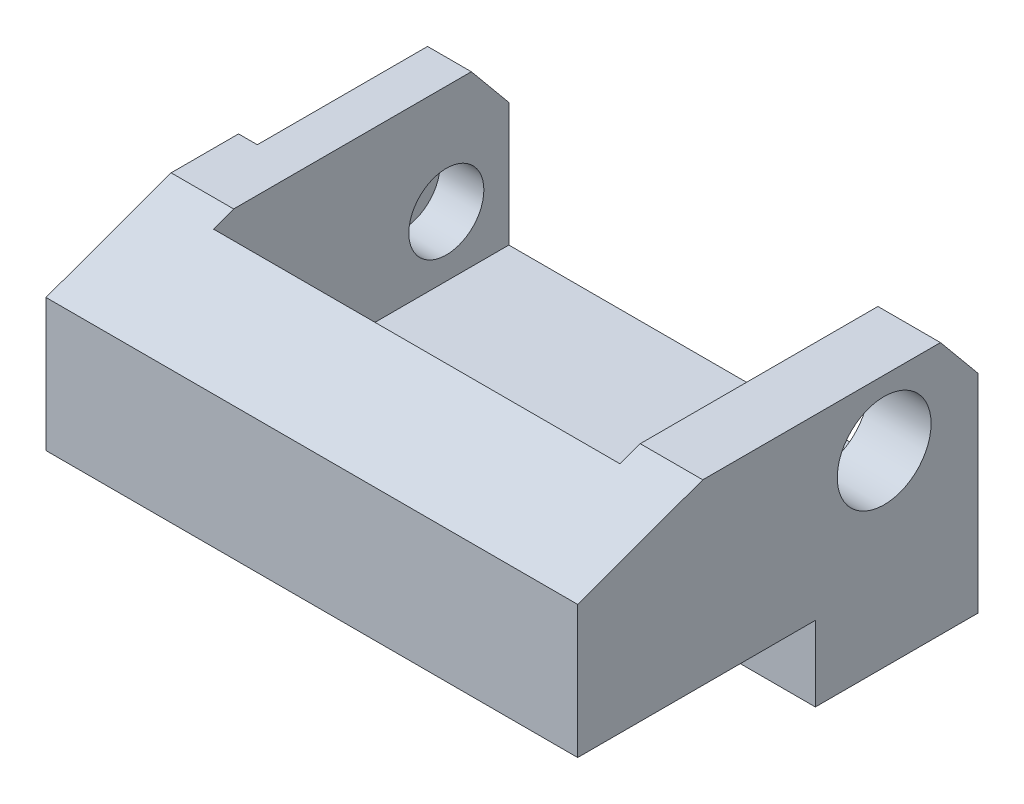
ISO-10303-21;
HEADER;
FILE_DESCRIPTION(('STEP AP214'),'2;1');
FILE_NAME('part.step','',(''),(''),'','','');
FILE_SCHEMA(('AUTOMOTIVE_DESIGN { 1 0 10303 214 1 1 1 1 }'));
ENDSEC;
DATA;
#1=APPLICATION_CONTEXT('core data for automotive mechanical design processes');
#2=APPLICATION_PROTOCOL_DEFINITION('international standard','automotive_design',2000,#1);
#3=PRODUCT_CONTEXT('',#1,'mechanical');
#4=PRODUCT('Part','Part','',(#3));
#5=PRODUCT_RELATED_PRODUCT_CATEGORY('part','',(#4));
#6=PRODUCT_DEFINITION_FORMATION('','',#4);
#7=PRODUCT_DEFINITION_CONTEXT('part definition',#1,'design');
#8=PRODUCT_DEFINITION('design','',#6,#7);
#9=PRODUCT_DEFINITION_SHAPE('','',#8);
#10=(LENGTH_UNIT() NAMED_UNIT(*) SI_UNIT(.MILLI.,.METRE.));
#11=(NAMED_UNIT(*) PLANE_ANGLE_UNIT() SI_UNIT($,.RADIAN.));
#12=(NAMED_UNIT(*) SI_UNIT($,.STERADIAN.) SOLID_ANGLE_UNIT());
#13=UNCERTAINTY_MEASURE_WITH_UNIT(LENGTH_MEASURE(1.E-05),#10,'distance_accuracy_value','');
#14=(GEOMETRIC_REPRESENTATION_CONTEXT(3) GLOBAL_UNCERTAINTY_ASSIGNED_CONTEXT((#13)) GLOBAL_UNIT_ASSIGNED_CONTEXT((#10,
#11,#12)) REPRESENTATION_CONTEXT('',''));
#15=CARTESIAN_POINT('',(0.,0.,0.));
#16=DIRECTION('',(0.,0.,1.));
#17=DIRECTION('',(1.,0.,0.));
#18=AXIS2_PLACEMENT_3D('',#15,#16,#17);
#19=CARTESIAN_POINT('',(42.5,21.206684421918,-64.));
#20=DIRECTION('',(0.,-0.637461940418098,0.770481845677362));
#21=DIRECTION('',(0.,-0.770481845677362,-0.637461940418098));
#22=AXIS2_PLACEMENT_3D('',#19,#20,#21);
#23=PLANE('',#22);
#24=DIRECTION('',(-1.,0.,0.));
#25=VECTOR('',#24,1.);
#26=CARTESIAN_POINT('',(42.5,21.206684421918,-64.));
#27=LINE('',#26,#25);
#28=CARTESIAN_POINT('',(-32.5,21.206684421918,-64.));
#29=VERTEX_POINT('',#28);
#30=CARTESIAN_POINT('',(-39.5,21.206684421918,-64.));
#31=VERTEX_POINT('',#30);
#32=EDGE_CURVE('E283',#29,#31,#27,.T.);
#33=ORIENTED_EDGE('',*,*,#32,.T.);
#34=DIRECTION('',(0.,-0.770481845677362,-0.637461940418098));
#35=VECTOR('',#34,1.);
#36=CARTESIAN_POINT('',(-39.5,40.0512826004509,-48.4088291129999));
#37=LINE('',#36,#35);
#38=CARTESIAN_POINT('',(-39.5,28.4587112190505,-58.));
#39=VERTEX_POINT('',#38);
#40=EDGE_CURVE('E197',#39,#31,#37,.T.);
#41=ORIENTED_EDGE('',*,*,#40,.F.);
#42=DIRECTION('',(-1.,0.,0.));
#43=VECTOR('',#42,1.);
#44=CARTESIAN_POINT('',(42.5,28.4587112190505,-58.));
#45=LINE('',#44,#43);
#46=CARTESIAN_POINT('',(-32.5,28.4587112190505,-58.));
#47=VERTEX_POINT('',#46);
#48=EDGE_CURVE('E278',#47,#39,#45,.T.);
#49=ORIENTED_EDGE('',*,*,#48,.F.);
#50=DIRECTION('',(0.,0.770481845677362,0.637461940418098));
#51=VECTOR('',#50,1.);
#52=CARTESIAN_POINT('',(-32.5,21.206684421918,-64.));
#53=LINE('',#52,#51);
#54=EDGE_CURVE('E236',#29,#47,#53,.T.);
#55=ORIENTED_EDGE('',*,*,#54,.F.);
#56=EDGE_LOOP('',(#33,#41,#49,#55));
#57=FACE_BOUND('',#56,.T.);
#58=ADVANCED_FACE('F41',(#57),#23,.F.);
#59=CARTESIAN_POINT('',(-39.5,28.0911505138034,-47.7793899312878));
#60=DIRECTION('',(-1.,0.,0.));
#61=DIRECTION('',(0.,0.,1.));
#62=AXIS2_PLACEMENT_3D('',#59,#60,#61);
#63=CYLINDRICAL_SURFACE('',#62,17.);
#64=CARTESIAN_POINT('',(-39.5,28.0911505138034,-47.7793899312878));
#65=DIRECTION('',(-1.,0.,0.));
#66=DIRECTION('',(0.,0.,1.));
#67=AXIS2_PLACEMENT_3D('',#64,#65,#66);
#68=CIRCLE('',#67,17.);
#69=CARTESIAN_POINT('',(-39.5,28.4587112190505,-30.7833639508429));
#70=VERTEX_POINT('',#69);
#71=CARTESIAN_POINT('',(-39.5,11.0911505138034,-47.7793899312878));
#72=VERTEX_POINT('',#71);
#73=EDGE_CURVE('E191',#70,#72,#68,.F.);
#74=ORIENTED_EDGE('',*,*,#73,.T.);
#75=DIRECTION('',(-1.,0.,0.));
#76=VECTOR('',#75,1.);
#77=CARTESIAN_POINT('',(-39.5,11.0911505138034,-47.7793899312876));
#78=LINE('',#77,#76);
#79=CARTESIAN_POINT('',(-42.5,11.0911505138034,-47.7793899312876));
#80=VERTEX_POINT('',#79);
#81=EDGE_CURVE('E181',#72,#80,#78,.T.);
#82=ORIENTED_EDGE('',*,*,#81,.T.);
#83=CARTESIAN_POINT('',(-42.5,28.0911505138034,-47.7793899312878));
#84=DIRECTION('',(-1.,0.,0.));
#85=DIRECTION('',(0.,0.,1.));
#86=AXIS2_PLACEMENT_3D('',#83,#84,#85);
#87=CIRCLE('',#86,17.);
#88=CARTESIAN_POINT('',(-42.5,28.4587112190505,-30.7833639508429));
#89=VERTEX_POINT('',#88);
#90=EDGE_CURVE('E192',#89,#80,#87,.F.);
#91=ORIENTED_EDGE('',*,*,#90,.F.);
#92=DIRECTION('',(-1.,0.,0.));
#93=VECTOR('',#92,1.);
#94=CARTESIAN_POINT('',(-39.5,28.4587112190505,-30.7833639508429));
#95=LINE('',#94,#93);
#96=EDGE_CURVE('E199',#70,#89,#95,.T.);
#97=ORIENTED_EDGE('',*,*,#96,.F.);
#98=EDGE_LOOP('',(#74,#82,#91,#97));
#99=FACE_BOUND('',#98,.T.);
#100=ADVANCED_FACE('F377',(#99),#63,.F.);
#101=CARTESIAN_POINT('',(42.5,28.4587112190505,-58.));
#102=DIRECTION('',(0.,-1.,0.));
#103=DIRECTION('',(0.,0.,-1.));
#104=AXIS2_PLACEMENT_3D('',#101,#102,#103);
#105=PLANE('',#104);
#106=ORIENTED_EDGE('',*,*,#96,.T.);
#107=DIRECTION('',(0.,0.,1.));
#108=VECTOR('',#107,1.);
#109=CARTESIAN_POINT('',(-42.5,28.4587112190505,-58.));
#110=LINE('',#109,#108);
#111=CARTESIAN_POINT('',(-42.5,28.4587112190505,-20.));
#112=VERTEX_POINT('',#111);
#113=EDGE_CURVE('E272',#89,#112,#110,.T.);
#114=ORIENTED_EDGE('',*,*,#113,.T.);
#115=DIRECTION('',(-1.,0.,0.));
#116=VECTOR('',#115,1.);
#117=CARTESIAN_POINT('',(42.5,28.4587112190505,-20.));
#118=LINE('',#117,#116);
#119=CARTESIAN_POINT('',(-32.5,28.4587112190505,-20.));
#120=VERTEX_POINT('',#119);
#121=EDGE_CURVE('E277',#120,#112,#118,.T.);
#122=ORIENTED_EDGE('',*,*,#121,.F.);
#123=DIRECTION('',(0.,0.,-1.));
#124=VECTOR('',#123,1.);
#125=CARTESIAN_POINT('',(-32.5,28.4587112190505,-16.7684012581446));
#126=LINE('',#125,#124);
#127=EDGE_CURVE('E216',#120,#47,#126,.T.);
#128=ORIENTED_EDGE('',*,*,#127,.T.);
#129=ORIENTED_EDGE('',*,*,#48,.T.);
#130=DIRECTION('',(0.,0.,-1.));
#131=VECTOR('',#130,1.);
#132=CARTESIAN_POINT('',(-39.5,28.4587112190505,0.));
#133=LINE('',#132,#131);
#134=EDGE_CURVE('E196',#70,#39,#133,.T.);
#135=ORIENTED_EDGE('',*,*,#134,.F.);
#136=EDGE_LOOP('',(#106,#114,#122,#128,#129,#135));
#137=FACE_BOUND('',#136,.T.);
#138=ADVANCED_FACE('F347',(#137),#105,.F.);
#139=CARTESIAN_POINT('',(-42.5,0.,0.));
#140=DIRECTION('',(1.,0.,0.));
#141=DIRECTION('',(0.,0.,-1.));
#142=AXIS2_PLACEMENT_3D('',#139,#140,#141);
#143=PLANE('',#142);
#144=ORIENTED_EDGE('',*,*,#90,.T.);
#145=DIRECTION('',(0.,0.,1.));
#146=VECTOR('',#145,1.);
#147=CARTESIAN_POINT('',(-42.5,11.0911505138034,-47.7793899312876));
#148=LINE('',#147,#146);
#149=CARTESIAN_POINT('',(-42.5,11.0911505138034,-64.));
#150=VERTEX_POINT('',#149);
#151=EDGE_CURVE('E183',#150,#80,#148,.T.);
#152=ORIENTED_EDGE('',*,*,#151,.F.);
#153=DIRECTION('',(0.,1.,0.));
#154=VECTOR('',#153,1.);
#155=CARTESIAN_POINT('',(-42.5,-12.,-64.));
#156=LINE('',#155,#154);
#157=CARTESIAN_POINT('',(-42.5,-12.,-64.));
#158=VERTEX_POINT('',#157);
#159=EDGE_CURVE('E270',#158,#150,#156,.T.);
#160=ORIENTED_EDGE('',*,*,#159,.F.);
#161=DIRECTION('',(0.,0.,-1.));
#162=VECTOR('',#161,1.);
#163=CARTESIAN_POINT('',(-42.5,-12.,-38.));
#164=LINE('',#163,#162);
#165=CARTESIAN_POINT('',(-42.5,-12.,-38.));
#166=VERTEX_POINT('',#165);
#167=EDGE_CURVE('E267',#166,#158,#164,.T.);
#168=ORIENTED_EDGE('',*,*,#167,.F.);
#169=DIRECTION('',(0.,-1.,0.));
#170=VECTOR('',#169,1.);
#171=CARTESIAN_POINT('',(-42.5,0.,-38.));
#172=LINE('',#171,#170);
#173=CARTESIAN_POINT('',(-42.5,0.,-38.));
#174=VERTEX_POINT('',#173);
#175=EDGE_CURVE('E263',#174,#166,#172,.T.);
#176=ORIENTED_EDGE('',*,*,#175,.F.);
#177=DIRECTION('',(0.,0.,-1.));
#178=VECTOR('',#177,1.);
#179=CARTESIAN_POINT('',(-42.5,0.,0.));
#180=LINE('',#179,#178);
#181=CARTESIAN_POINT('',(-42.5,0.,0.));
#182=VERTEX_POINT('',#181);
#183=EDGE_CURVE('E265',#182,#174,#180,.T.);
#184=ORIENTED_EDGE('',*,*,#183,.F.);
#185=DIRECTION('',(0.,-1.,0.));
#186=VECTOR('',#185,1.);
#187=CARTESIAN_POINT('',(-42.5,21.206684421918,0.));
#188=LINE('',#187,#186);
#189=CARTESIAN_POINT('',(-42.5,21.206684421918,0.));
#190=VERTEX_POINT('',#189);
#191=EDGE_CURVE('E239',#190,#182,#188,.T.);
#192=ORIENTED_EDGE('',*,*,#191,.F.);
#193=DIRECTION('',(0.,-0.3408835273402,0.940105537047891));
#194=VECTOR('',#193,1.);
#195=CARTESIAN_POINT('',(-42.5,28.4587112190505,-20.));
#196=LINE('',#195,#194);
#197=EDGE_CURVE('E244',#112,#190,#196,.T.);
#198=ORIENTED_EDGE('',*,*,#197,.F.);
#199=ORIENTED_EDGE('',*,*,#113,.F.);
#200=EDGE_LOOP('',(#144,#152,#160,#168,#176,#184,#192,#198,#199));
#201=FACE_BOUND('',#200,.T.);
#202=ADVANCED_FACE('F351',(#201),#143,.F.);
#203=CARTESIAN_POINT('',(42.5,-12.,-64.));
#204=DIRECTION('',(0.,0.,1.));
#205=DIRECTION('',(1.,0.,0.));
#206=AXIS2_PLACEMENT_3D('',#203,#204,#205);
#207=PLANE('',#206);
#208=ORIENTED_EDGE('',*,*,#159,.T.);
#209=DIRECTION('',(-1.,0.,0.));
#210=VECTOR('',#209,1.);
#211=CARTESIAN_POINT('',(-39.5,11.0911505138034,-64.));
#212=LINE('',#211,#210);
#213=CARTESIAN_POINT('',(-39.5,11.0911505138034,-64.));
#214=VERTEX_POINT('',#213);
#215=EDGE_CURVE('E190',#214,#150,#212,.T.);
#216=ORIENTED_EDGE('',*,*,#215,.F.);
#217=DIRECTION('',(0.,-1.,0.));
#218=VECTOR('',#217,1.);
#219=CARTESIAN_POINT('',(-39.5,11.0911505138034,-64.));
#220=LINE('',#219,#218);
#221=EDGE_CURVE('E182',#31,#214,#220,.T.);
#222=ORIENTED_EDGE('',*,*,#221,.F.);
#223=ORIENTED_EDGE('',*,*,#32,.F.);
#224=DIRECTION('',(0.,1.,0.));
#225=VECTOR('',#224,1.);
#226=CARTESIAN_POINT('',(-32.5,-12.,-64.));
#227=LINE('',#226,#225);
#228=CARTESIAN_POINT('',(-32.5,1.45871121905055,-64.));
#229=VERTEX_POINT('',#228);
#230=EDGE_CURVE('E238',#229,#29,#227,.T.);
#231=ORIENTED_EDGE('',*,*,#230,.F.);
#232=DIRECTION('',(-1.,0.,0.));
#233=VECTOR('',#232,1.);
#234=CARTESIAN_POINT('',(42.5,1.45871121905055,-64.));
#235=LINE('',#234,#233);
#236=CARTESIAN_POINT('',(32.5,1.45871121905055,-64.));
#237=VERTEX_POINT('',#236);
#238=EDGE_CURVE('E11',#237,#229,#235,.T.);
#239=ORIENTED_EDGE('',*,*,#238,.F.);
#240=DIRECTION('',(0.,1.,0.));
#241=VECTOR('',#240,1.);
#242=CARTESIAN_POINT('',(32.5,-12.,-64.));
#243=LINE('',#242,#241);
#244=CARTESIAN_POINT('',(32.5,21.206684421918,-64.));
#245=VERTEX_POINT('',#244);
#246=EDGE_CURVE('E231',#237,#245,#243,.T.);
#247=ORIENTED_EDGE('',*,*,#246,.T.);
#248=CARTESIAN_POINT('',(42.5,21.206684421918,-64.));
#249=VERTEX_POINT('',#248);
#250=EDGE_CURVE('E284',#249,#245,#27,.T.);
#251=ORIENTED_EDGE('',*,*,#250,.F.);
#252=DIRECTION('',(0.,1.,0.));
#253=VECTOR('',#252,1.);
#254=CARTESIAN_POINT('',(42.5,-12.,-64.));
#255=LINE('',#254,#253);
#256=CARTESIAN_POINT('',(42.5,-12.,-64.));
#257=VERTEX_POINT('',#256);
#258=EDGE_CURVE('E252',#257,#249,#255,.T.);
#259=ORIENTED_EDGE('',*,*,#258,.F.);
#260=DIRECTION('',(-1.,0.,0.));
#261=VECTOR('',#260,1.);
#262=CARTESIAN_POINT('',(42.5,-12.,-64.));
#263=LINE('',#262,#261);
#264=EDGE_CURVE('E290',#257,#158,#263,.T.);
#265=ORIENTED_EDGE('',*,*,#264,.T.);
#266=EDGE_LOOP('',(#208,#216,#222,#223,#231,#239,#247,#251,#259,#265));
#267=FACE_BOUND('',#266,.T.);
#268=ADVANCED_FACE('F335',(#267),#207,.F.);
#269=CARTESIAN_POINT('',(42.5,28.4587112190505,-20.));
#270=DIRECTION('',(0.,-0.940105537047891,-0.3408835273402));
#271=DIRECTION('',(0.,0.3408835273402,-0.940105537047891));
#272=AXIS2_PLACEMENT_3D('',#269,#270,#271);
#273=PLANE('',#272);
#274=DIRECTION('',(0.,-0.3408835273402,0.940105537047891));
#275=VECTOR('',#274,1.);
#276=CARTESIAN_POINT('',(-32.5,28.4587112190505,-20.));
#277=LINE('',#276,#275);
#278=CARTESIAN_POINT('',(-32.5,27.2869291853748,-16.7684012581446));
#279=VERTEX_POINT('',#278);
#280=EDGE_CURVE('E47',#120,#279,#277,.T.);
#281=ORIENTED_EDGE('',*,*,#280,.F.);
#282=ORIENTED_EDGE('',*,*,#121,.T.);
#283=ORIENTED_EDGE('',*,*,#197,.T.);
#284=DIRECTION('',(-1.,0.,0.));
#285=VECTOR('',#284,1.);
#286=CARTESIAN_POINT('',(42.5,21.206684421918,0.));
#287=LINE('',#286,#285);
#288=CARTESIAN_POINT('',(42.5,21.206684421918,0.));
#289=VERTEX_POINT('',#288);
#290=EDGE_CURVE('E256',#289,#190,#287,.T.);
#291=ORIENTED_EDGE('',*,*,#290,.F.);
#292=DIRECTION('',(0.,-0.3408835273402,0.940105537047891));
#293=VECTOR('',#292,1.);
#294=CARTESIAN_POINT('',(42.5,28.4587112190505,-20.));
#295=LINE('',#294,#293);
#296=CARTESIAN_POINT('',(42.5,28.4587112190505,-20.));
#297=VERTEX_POINT('',#296);
#298=EDGE_CURVE('E260',#297,#289,#295,.T.);
#299=ORIENTED_EDGE('',*,*,#298,.F.);
#300=CARTESIAN_POINT('',(32.5,28.4587112190505,-20.));
#301=VERTEX_POINT('',#300);
#302=EDGE_CURVE('E280',#297,#301,#118,.T.);
#303=ORIENTED_EDGE('',*,*,#302,.T.);
#304=DIRECTION('',(0.,-0.3408835273402,0.940105537047891));
#305=VECTOR('',#304,1.);
#306=CARTESIAN_POINT('',(32.5,28.4587112190505,-20.));
#307=LINE('',#306,#305);
#308=CARTESIAN_POINT('',(32.5,27.2869291853748,-16.7684012581447));
#309=VERTEX_POINT('',#308);
#310=EDGE_CURVE('E297',#301,#309,#307,.T.);
#311=ORIENTED_EDGE('',*,*,#310,.T.);
#312=DIRECTION('',(-1.,0.,0.));
#313=VECTOR('',#312,1.);
#314=CARTESIAN_POINT('',(42.5,27.2869291853748,-16.7684012581447));
#315=LINE('',#314,#313);
#316=EDGE_CURVE('E303',#309,#279,#315,.T.);
#317=ORIENTED_EDGE('',*,*,#316,.T.);
#318=EDGE_LOOP('',(#281,#282,#283,#291,#299,#303,#311,#317));
#319=FACE_BOUND('',#318,.T.);
#320=ADVANCED_FACE('F317',(#319),#273,.F.);
#321=CARTESIAN_POINT('',(42.5,21.206684421918,0.));
#322=DIRECTION('',(0.,0.,-1.));
#323=DIRECTION('',(-1.,0.,0.));
#324=AXIS2_PLACEMENT_3D('',#321,#322,#323);
#325=PLANE('',#324);
#326=ORIENTED_EDGE('',*,*,#191,.T.);
#327=DIRECTION('',(-1.,0.,0.));
#328=VECTOR('',#327,1.);
#329=CARTESIAN_POINT('',(42.5,0.,0.));
#330=LINE('',#329,#328);
#331=CARTESIAN_POINT('',(42.5,0.,0.));
#332=VERTEX_POINT('',#331);
#333=EDGE_CURVE('E300',#332,#182,#330,.T.);
#334=ORIENTED_EDGE('',*,*,#333,.F.);
#335=DIRECTION('',(0.,-1.,0.));
#336=VECTOR('',#335,1.);
#337=CARTESIAN_POINT('',(42.5,21.206684421918,0.));
#338=LINE('',#337,#336);
#339=EDGE_CURVE('E241',#289,#332,#338,.T.);
#340=ORIENTED_EDGE('',*,*,#339,.F.);
#341=ORIENTED_EDGE('',*,*,#290,.T.);
#342=EDGE_LOOP('',(#326,#334,#340,#341));
#343=FACE_BOUND('',#342,.T.);
#344=ADVANCED_FACE('F43',(#343),#325,.F.);
#345=CARTESIAN_POINT('',(42.5,0.,0.));
#346=DIRECTION('',(0.,1.,0.));
#347=DIRECTION('',(0.,0.,1.));
#348=AXIS2_PLACEMENT_3D('',#345,#346,#347);
#349=PLANE('',#348);
#350=ORIENTED_EDGE('',*,*,#183,.T.);
#351=DIRECTION('',(-1.,0.,0.));
#352=VECTOR('',#351,1.);
#353=CARTESIAN_POINT('',(42.5,0.,-38.));
#354=LINE('',#353,#352);
#355=CARTESIAN_POINT('',(42.5,0.,-38.));
#356=VERTEX_POINT('',#355);
#357=EDGE_CURVE('E295',#356,#174,#354,.T.);
#358=ORIENTED_EDGE('',*,*,#357,.F.);
#359=DIRECTION('',(0.,0.,-1.));
#360=VECTOR('',#359,1.);
#361=CARTESIAN_POINT('',(42.5,0.,0.));
#362=LINE('',#361,#360);
#363=EDGE_CURVE('E242',#332,#356,#362,.T.);
#364=ORIENTED_EDGE('',*,*,#363,.F.);
#365=ORIENTED_EDGE('',*,*,#333,.T.);
#366=EDGE_LOOP('',(#350,#358,#364,#365));
#367=FACE_BOUND('',#366,.T.);
#368=ADVANCED_FACE('F398',(#367),#349,.F.);
#369=CARTESIAN_POINT('',(42.5,0.,-38.));
#370=DIRECTION('',(0.,0.,-1.));
#371=DIRECTION('',(-1.,0.,0.));
#372=AXIS2_PLACEMENT_3D('',#369,#370,#371);
#373=PLANE('',#372);
#374=ORIENTED_EDGE('',*,*,#175,.T.);
#375=DIRECTION('',(-1.,0.,0.));
#376=VECTOR('',#375,1.);
#377=CARTESIAN_POINT('',(42.5,-12.,-38.));
#378=LINE('',#377,#376);
#379=CARTESIAN_POINT('',(42.5,-12.,-38.));
#380=VERTEX_POINT('',#379);
#381=EDGE_CURVE('E293',#380,#166,#378,.T.);
#382=ORIENTED_EDGE('',*,*,#381,.F.);
#383=DIRECTION('',(0.,-1.,0.));
#384=VECTOR('',#383,1.);
#385=CARTESIAN_POINT('',(42.5,0.,-38.));
#386=LINE('',#385,#384);
#387=EDGE_CURVE('E250',#356,#380,#386,.T.);
#388=ORIENTED_EDGE('',*,*,#387,.F.);
#389=ORIENTED_EDGE('',*,*,#357,.T.);
#390=EDGE_LOOP('',(#374,#382,#388,#389));
#391=FACE_BOUND('',#390,.T.);
#392=ADVANCED_FACE('F394',(#391),#373,.F.);
#393=CARTESIAN_POINT('',(42.5,-12.,-38.));
#394=DIRECTION('',(0.,1.,0.));
#395=DIRECTION('',(0.,0.,1.));
#396=AXIS2_PLACEMENT_3D('',#393,#394,#395);
#397=PLANE('',#396);
#398=ORIENTED_EDGE('',*,*,#167,.T.);
#399=ORIENTED_EDGE('',*,*,#264,.F.);
#400=DIRECTION('',(0.,0.,-1.));
#401=VECTOR('',#400,1.);
#402=CARTESIAN_POINT('',(42.5,-12.,-38.));
#403=LINE('',#402,#401);
#404=EDGE_CURVE('E248',#380,#257,#403,.T.);
#405=ORIENTED_EDGE('',*,*,#404,.F.);
#406=ORIENTED_EDGE('',*,*,#381,.T.);
#407=EDGE_LOOP('',(#398,#399,#405,#406));
#408=FACE_BOUND('',#407,.T.);
#409=ADVANCED_FACE('F386',(#408),#397,.F.);
#410=ORIENTED_EDGE('',*,*,#250,.T.);
#411=DIRECTION('',(0.,0.770481845677362,0.637461940418098));
#412=VECTOR('',#411,1.);
#413=CARTESIAN_POINT('',(32.5,21.206684421918,-64.));
#414=LINE('',#413,#412);
#415=CARTESIAN_POINT('',(32.5,28.4587112190505,-58.));
#416=VERTEX_POINT('',#415);
#417=EDGE_CURVE('E230',#245,#416,#414,.T.);
#418=ORIENTED_EDGE('',*,*,#417,.T.);
#419=CARTESIAN_POINT('',(42.5,28.4587112190505,-58.));
#420=VERTEX_POINT('',#419);
#421=EDGE_CURVE('E281',#420,#416,#45,.T.);
#422=ORIENTED_EDGE('',*,*,#421,.F.);
#423=DIRECTION('',(0.,0.770481845677362,0.637461940418098));
#424=VECTOR('',#423,1.);
#425=CARTESIAN_POINT('',(42.5,21.206684421918,-64.));
#426=LINE('',#425,#424);
#427=EDGE_CURVE('E254',#249,#420,#426,.T.);
#428=ORIENTED_EDGE('',*,*,#427,.F.);
#429=EDGE_LOOP('',(#410,#418,#422,#428));
#430=FACE_BOUND('',#429,.T.);
#431=ADVANCED_FACE('F328',(#430),#23,.F.);
#432=ORIENTED_EDGE('',*,*,#421,.T.);
#433=DIRECTION('',(0.,0.,-1.));
#434=VECTOR('',#433,1.);
#435=CARTESIAN_POINT('',(32.5,28.4587112190505,-16.7684012581447));
#436=LINE('',#435,#434);
#437=EDGE_CURVE('E212',#301,#416,#436,.T.);
#438=ORIENTED_EDGE('',*,*,#437,.F.);
#439=ORIENTED_EDGE('',*,*,#302,.F.);
#440=DIRECTION('',(0.,0.,1.));
#441=VECTOR('',#440,1.);
#442=CARTESIAN_POINT('',(42.5,28.4587112190505,-58.));
#443=LINE('',#442,#441);
#444=EDGE_CURVE('E253',#420,#297,#443,.T.);
#445=ORIENTED_EDGE('',*,*,#444,.F.);
#446=EDGE_LOOP('',(#432,#438,#439,#445));
#447=FACE_BOUND('',#446,.T.);
#448=ADVANCED_FACE('F321',(#447),#105,.F.);
#449=CARTESIAN_POINT('',(42.5,0.,0.));
#450=DIRECTION('',(1.,0.,0.));
#451=DIRECTION('',(0.,0.,-1.));
#452=AXIS2_PLACEMENT_3D('',#449,#450,#451);
#453=PLANE('',#452);
#454=CARTESIAN_POINT('',(42.5,18.,-49.));
#455=DIRECTION('',(1.,0.,0.));
#456=DIRECTION('',(0.,0.,-1.));
#457=AXIS2_PLACEMENT_3D('',#454,#455,#456);
#458=CIRCLE('',#457,7.5);
#459=CARTESIAN_POINT('',(42.5,18.,-56.5));
#460=VERTEX_POINT('',#459);
#461=EDGE_CURVE('E203',#460,#460,#458,.T.);
#462=ORIENTED_EDGE('',*,*,#461,.F.);
#463=EDGE_LOOP('',(#462));
#464=FACE_BOUND('',#463,.T.);
#465=ORIENTED_EDGE('',*,*,#339,.T.);
#466=ORIENTED_EDGE('',*,*,#363,.T.);
#467=ORIENTED_EDGE('',*,*,#387,.T.);
#468=ORIENTED_EDGE('',*,*,#404,.T.);
#469=ORIENTED_EDGE('',*,*,#258,.T.);
#470=ORIENTED_EDGE('',*,*,#427,.T.);
#471=ORIENTED_EDGE('',*,*,#444,.T.);
#472=ORIENTED_EDGE('',*,*,#298,.T.);
#473=EDGE_LOOP('',(#465,#466,#467,#468,#469,#470,#471,#472));
#474=FACE_BOUND('',#473,.T.);
#475=ADVANCED_FACE('F359',(#464,#474),#453,.T.);
#476=CARTESIAN_POINT('',(0.,1.45871121905054,0.));
#477=DIRECTION('',(0.,1.,0.));
#478=DIRECTION('',(0.,0.,1.));
#479=AXIS2_PLACEMENT_3D('',#476,#477,#478);
#480=PLANE('',#479);
#481=ORIENTED_EDGE('',*,*,#238,.T.);
#482=DIRECTION('',(0.,0.,-1.));
#483=VECTOR('',#482,1.);
#484=CARTESIAN_POINT('',(-32.5,1.45871121905054,-16.7684012581447));
#485=LINE('',#484,#483);
#486=CARTESIAN_POINT('',(-32.5,1.45871121905054,-16.7684012581447));
#487=VERTEX_POINT('',#486);
#488=EDGE_CURVE('E218',#487,#229,#485,.T.);
#489=ORIENTED_EDGE('',*,*,#488,.F.);
#490=DIRECTION('',(1.,0.,0.));
#491=VECTOR('',#490,1.);
#492=CARTESIAN_POINT('',(-32.5,1.45871121905054,-16.7684012581447));
#493=LINE('',#492,#491);
#494=CARTESIAN_POINT('',(32.5,1.45871121905054,-16.7684012581447));
#495=VERTEX_POINT('',#494);
#496=EDGE_CURVE('E215',#487,#495,#493,.T.);
#497=ORIENTED_EDGE('',*,*,#496,.T.);
#498=DIRECTION('',(0.,0.,-1.));
#499=VECTOR('',#498,1.);
#500=CARTESIAN_POINT('',(32.5,1.45871121905054,-16.7684012581447));
#501=LINE('',#500,#499);
#502=EDGE_CURVE('E213',#495,#237,#501,.T.);
#503=ORIENTED_EDGE('',*,*,#502,.T.);
#504=EDGE_LOOP('',(#481,#489,#497,#503));
#505=FACE_BOUND('',#504,.T.);
#506=ADVANCED_FACE('F336',(#505),#480,.T.);
#507=CARTESIAN_POINT('',(-32.5,1.45871121905054,-16.7684012581447));
#508=DIRECTION('',(0.,0.,1.));
#509=DIRECTION('',(1.,0.,0.));
#510=AXIS2_PLACEMENT_3D('',#507,#508,#509);
#511=PLANE('',#510);
#512=DIRECTION('',(0.,1.,0.));
#513=VECTOR('',#512,1.);
#514=CARTESIAN_POINT('',(32.5,1.45871121905054,-16.7684012581447));
#515=LINE('',#514,#513);
#516=EDGE_CURVE('E224',#495,#309,#515,.T.);
#517=ORIENTED_EDGE('',*,*,#516,.F.);
#518=ORIENTED_EDGE('',*,*,#496,.F.);
#519=DIRECTION('',(0.,1.,0.));
#520=VECTOR('',#519,1.);
#521=CARTESIAN_POINT('',(-32.5,1.45871121905054,-16.7684012581447));
#522=LINE('',#521,#520);
#523=EDGE_CURVE('E228',#487,#279,#522,.T.);
#524=ORIENTED_EDGE('',*,*,#523,.T.);
#525=ORIENTED_EDGE('',*,*,#316,.F.);
#526=EDGE_LOOP('',(#517,#518,#524,#525));
#527=FACE_BOUND('',#526,.T.);
#528=ADVANCED_FACE('F314',(#527),#511,.F.);
#529=CARTESIAN_POINT('',(-32.5,1.45871121905054,-16.7684012581447));
#530=DIRECTION('',(1.,0.,0.));
#531=DIRECTION('',(0.,0.,-1.));
#532=AXIS2_PLACEMENT_3D('',#529,#530,#531);
#533=PLANE('',#532);
#534=CARTESIAN_POINT('',(-32.5,11.0911505138034,-54.));
#535=DIRECTION('',(1.,0.,0.));
#536=DIRECTION('',(0.,0.,-1.));
#537=AXIS2_PLACEMENT_3D('',#534,#535,#536);
#538=CIRCLE('',#537,5.99999999999999);
#539=CARTESIAN_POINT('',(-32.5,11.0911505138034,-60.));
#540=VERTEX_POINT('',#539);
#541=EDGE_CURVE('E178',#540,#540,#538,.F.);
#542=ORIENTED_EDGE('',*,*,#541,.T.);
#543=EDGE_LOOP('',(#542));
#544=FACE_BOUND('',#543,.T.);
#545=ORIENTED_EDGE('',*,*,#230,.T.);
#546=ORIENTED_EDGE('',*,*,#54,.T.);
#547=ORIENTED_EDGE('',*,*,#127,.F.);
#548=ORIENTED_EDGE('',*,*,#280,.T.);
#549=ORIENTED_EDGE('',*,*,#523,.F.);
#550=ORIENTED_EDGE('',*,*,#488,.T.);
#551=EDGE_LOOP('',(#545,#546,#547,#548,#549,#550));
#552=FACE_BOUND('',#551,.T.);
#553=ADVANCED_FACE('F310',(#544,#552),#533,.T.);
#554=CARTESIAN_POINT('',(32.5,1.45871121905054,-16.7684012581447));
#555=DIRECTION('',(1.,0.,0.));
#556=DIRECTION('',(0.,0.,-1.));
#557=AXIS2_PLACEMENT_3D('',#554,#555,#556);
#558=PLANE('',#557);
#559=CARTESIAN_POINT('',(32.5,18.,-49.));
#560=DIRECTION('',(1.,0.,0.));
#561=DIRECTION('',(0.,0.,-1.));
#562=AXIS2_PLACEMENT_3D('',#559,#560,#561);
#563=CIRCLE('',#562,7.5);
#564=CARTESIAN_POINT('',(32.5,18.,-56.5));
#565=VERTEX_POINT('',#564);
#566=EDGE_CURVE('E206',#565,#565,#563,.F.);
#567=ORIENTED_EDGE('',*,*,#566,.F.);
#568=EDGE_LOOP('',(#567));
#569=FACE_BOUND('',#568,.T.);
#570=ORIENTED_EDGE('',*,*,#502,.F.);
#571=ORIENTED_EDGE('',*,*,#516,.T.);
#572=ORIENTED_EDGE('',*,*,#310,.F.);
#573=ORIENTED_EDGE('',*,*,#437,.T.);
#574=ORIENTED_EDGE('',*,*,#417,.F.);
#575=ORIENTED_EDGE('',*,*,#246,.F.);
#576=EDGE_LOOP('',(#570,#571,#572,#573,#574,#575));
#577=FACE_BOUND('',#576,.T.);
#578=ADVANCED_FACE('F325',(#569,#577),#558,.F.);
#579=CARTESIAN_POINT('',(11.2867965644036,18.,-49.));
#580=DIRECTION('',(1.,0.,0.));
#581=DIRECTION('',(0.,0.,-1.));
#582=AXIS2_PLACEMENT_3D('',#579,#580,#581);
#583=CYLINDRICAL_SURFACE('',#582,7.5);
#584=ORIENTED_EDGE('',*,*,#566,.T.);
#585=EDGE_LOOP('',(#584));
#586=FACE_BOUND('',#585,.T.);
#587=ORIENTED_EDGE('',*,*,#461,.T.);
#588=EDGE_LOOP('',(#587));
#589=FACE_BOUND('',#588,.T.);
#590=ADVANCED_FACE('F430',(#586,#589),#583,.F.);
#591=CARTESIAN_POINT('',(-39.5,0.,0.));
#592=DIRECTION('',(-1.,0.,0.));
#593=DIRECTION('',(0.,0.,1.));
#594=AXIS2_PLACEMENT_3D('',#591,#592,#593);
#595=PLANE('',#594);
#596=CARTESIAN_POINT('',(-39.5,11.0911505138034,-54.));
#597=DIRECTION('',(-1.,0.,0.));
#598=DIRECTION('',(0.,0.,1.));
#599=AXIS2_PLACEMENT_3D('',#596,#597,#598);
#600=CIRCLE('',#599,5.99999999999999);
#601=CARTESIAN_POINT('',(-39.5,11.0911505138034,-48.));
#602=VERTEX_POINT('',#601);
#603=CARTESIAN_POINT('',(-39.5,11.0911505138034,-60.));
#604=VERTEX_POINT('',#603);
#605=EDGE_CURVE('E54',#602,#604,#600,.T.);
#606=ORIENTED_EDGE('',*,*,#605,.F.);
#607=DIRECTION('',(0.,0.,1.));
#608=VECTOR('',#607,1.);
#609=CARTESIAN_POINT('',(-39.5,11.0911505138034,-47.7793899312876));
#610=LINE('',#609,#608);
#611=EDGE_CURVE('E65',#602,#72,#610,.T.);
#612=ORIENTED_EDGE('',*,*,#611,.T.);
#613=ORIENTED_EDGE('',*,*,#73,.F.);
#614=ORIENTED_EDGE('',*,*,#134,.T.);
#615=ORIENTED_EDGE('',*,*,#40,.T.);
#616=ORIENTED_EDGE('',*,*,#221,.T.);
#617=EDGE_CURVE('E175',#214,#604,#610,.T.);
#618=ORIENTED_EDGE('',*,*,#617,.T.);
#619=EDGE_LOOP('',(#606,#612,#613,#614,#615,#616,#618));
#620=FACE_BOUND('',#619,.T.);
#621=ADVANCED_FACE('F180',(#620),#595,.T.);
#622=CARTESIAN_POINT('',(-39.5,11.0911505138034,-47.7793899312876));
#623=DIRECTION('',(0.,-1.,0.));
#624=DIRECTION('',(0.,0.,-1.));
#625=AXIS2_PLACEMENT_3D('',#622,#623,#624);
#626=PLANE('',#625);
#627=ORIENTED_EDGE('',*,*,#151,.T.);
#628=ORIENTED_EDGE('',*,*,#81,.F.);
#629=ORIENTED_EDGE('',*,*,#611,.F.);
#630=EDGE_CURVE('E168',#604,#602,#610,.T.);
#631=ORIENTED_EDGE('',*,*,#630,.F.);
#632=ORIENTED_EDGE('',*,*,#617,.F.);
#633=ORIENTED_EDGE('',*,*,#215,.T.);
#634=EDGE_LOOP('',(#627,#628,#629,#631,#632,#633));
#635=FACE_BOUND('',#634,.T.);
#636=ADVANCED_FACE('F177',(#635),#626,.F.);
#637=CARTESIAN_POINT('',(-39.5,11.0911505138034,-54.));
#638=DIRECTION('',(-1.,0.,0.));
#639=DIRECTION('',(0.,0.,1.));
#640=AXIS2_PLACEMENT_3D('',#637,#638,#639);
#641=PLANE('',#640);
#642=EDGE_CURVE('E166',#604,#602,#600,.T.);
#643=ORIENTED_EDGE('',*,*,#642,.F.);
#644=ORIENTED_EDGE('',*,*,#630,.T.);
#645=EDGE_LOOP('',(#643,#644));
#646=FACE_BOUND('',#645,.T.);
#647=ADVANCED_FACE('F170',(#646),#641,.F.);
#648=CARTESIAN_POINT('',(-15.5294372515229,11.0911505138034,-54.));
#649=DIRECTION('',(-1.,0.,0.));
#650=DIRECTION('',(0.,0.,1.));
#651=AXIS2_PLACEMENT_3D('',#648,#649,#650);
#652=CYLINDRICAL_SURFACE('',#651,5.99999999999999);
#653=ORIENTED_EDGE('',*,*,#605,.T.);
#654=ORIENTED_EDGE('',*,*,#642,.T.);
#655=EDGE_LOOP('',(#653,#654));
#656=FACE_BOUND('',#655,.T.);
#657=ORIENTED_EDGE('',*,*,#541,.F.);
#658=EDGE_LOOP('',(#657));
#659=FACE_BOUND('',#658,.T.);
#660=ADVANCED_FACE('F172',(#656,#659),#652,.F.);
#661=CLOSED_SHELL('',(#58,#100,#138,#202,#268,#320,#344,#368,#392,#409,#431,#448,#475,#506,#528,
#553,#578,#590,#621,#636,#647,#660));
#662=MANIFOLD_SOLID_BREP('B2',#661);
#663=ADVANCED_BREP_SHAPE_REPRESENTATION('',(#18,#662),#14);
#664=SHAPE_DEFINITION_REPRESENTATION(#9,#663);
ENDSEC;
END-ISO-10303-21;
